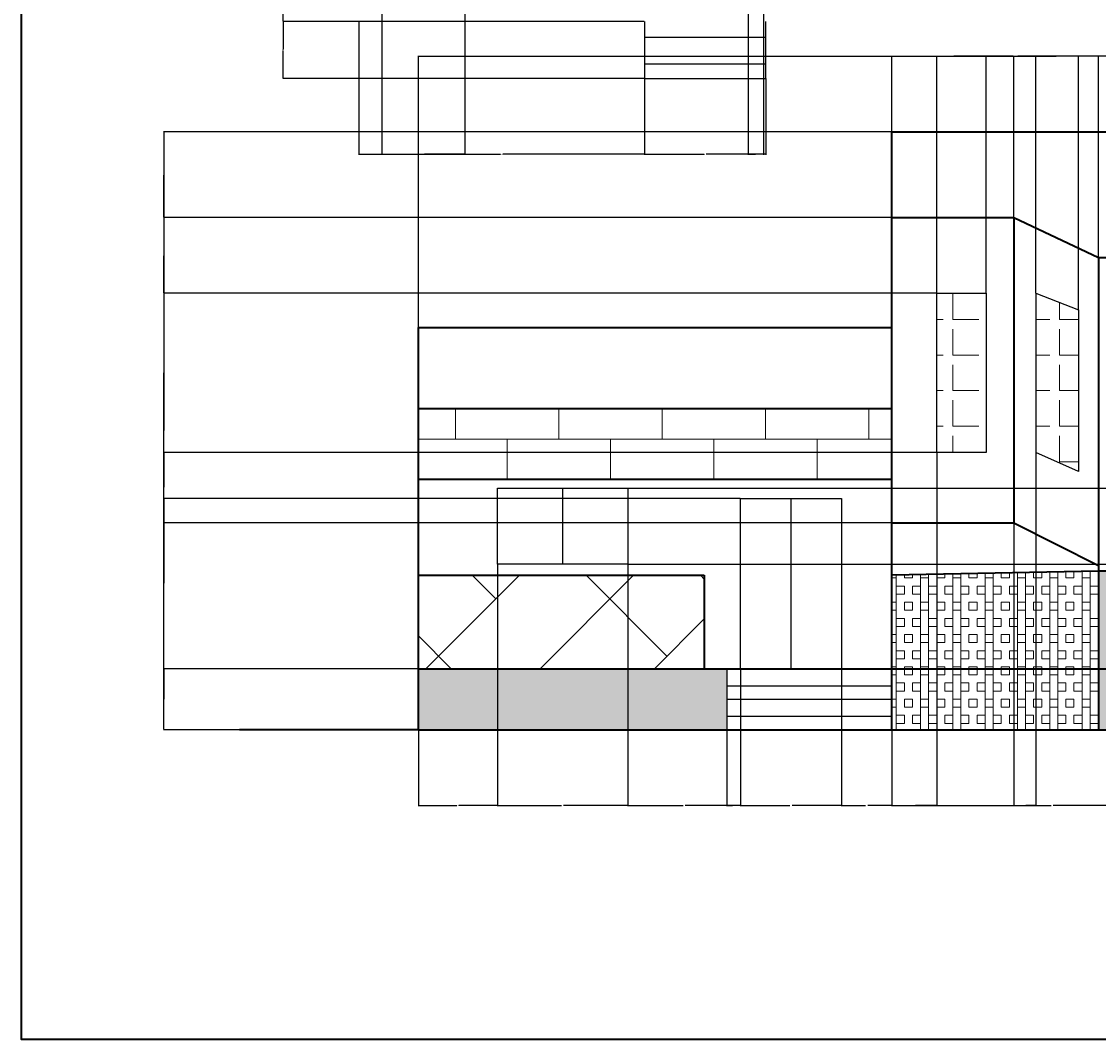
# Model space of a CAD drawing. Units: feet. Extents: x 3406 to 4127, y 2162 to 3204.
# Tile 1 of 3: x 3406 to 3829, y 2162 to 2562. Entities that reach past the tile are written whole.
import ezdxf

# ---------------------------------------------------------------- set-up
doc = ezdxf.new("R2010")
doc.units = ezdxf.units.FT
for name, color, linetype, lineweight in [('A-ANNO-DIMS', 2, 'Continuous', 18), ('A-ANNO-TTLB', 7, 'Continuous', 35), ('A-DOOR', 3, 'Continuous', 25), ('A-ELEV', 7, 'Continuous', 35), ('A-ELEV-GRND', 7, 'Continuous', 35), ('A-ELEV-PATT', 8, 'Continuous', 13), ('A-FLOR-STRS', 7, 'Continuous', 25), ('A-GLAZ', 4, 'Continuous', 25), ('A-GLAZ-PATT', 9, 'Continuous', 13)]:
    doc.layers.add(name, color=color, linetype=linetype, lineweight=lineweight)
doc.styles.get("Standard").update_dxf_attribs({"font": 'arial.ttf'})
doc.dimstyles.get("Standard").update_dxf_attribs({"dimtxt": 0.18, "dimasz": 0.18, "dimexe": 0.18, "dimexo": 0.0625, "dimgap": 0.09, "dimtad": 0, "dimtih": 1, "dimtoh": 1, "dimdec": 4, "dimzin": 0, "dimdsep": 46, "dimtxsty": 'Standard', "dimcen": 0.09, "dimadec": 0, "dimazin": 0, "dimtfac": 1, "dimtdec": 4, "dimtofl": 0, "dimtmove": 0, "dimatfit": 3, "dimfxl": 1, "dimtolj": 1, "dimtzin": 0, "dimarcsym": 0})

# ---------------------------------------------------------------- blocks, each defined once
blk = doc.blocks.new('*D5')
at = {"layer": 'A-ANNO-DIMS', "color": 0, "lineweight": -2, "transparency": 16777216}
for p, q in [((3538.33, 3101.91), (3508.41, 3101.91)), ((3508.59, 3101.73), (3508.59, 2832.09)), ((3508.59, 2562.09), (3508.59, 2831.72)), ((3538.33, 2561.91), (3508.41, 2561.91))]:
    blk.add_line(p, q, dxfattribs=at)
at = {"layer": 'A-ANNO-DIMS', "color": 0, "transparency": 16777216}
for points in [[(3508.56, 3101.73), (3508.62, 3101.73), (3508.59, 3101.91)], [(3508.56, 2562.09), (3508.62, 2562.09), (3508.59, 2561.91)]]:
    blk.add_solid(points, dxfattribs=at)
at = {"layer": 'Defpoints', "color": 0, "transparency": 16777216}
for p in [(3538.39, 3101.91), (3508.59, 2561.91), (3538.39, 2561.91)]:
    blk.add_point(p, dxfattribs=at)
at = {"layer": 'A-ANNO-DIMS', "color": 0, "transparency": 16777216, "insert": (3508.59, 2831.91), "char_height": 0.18, "attachment_point": 5}
blk.add_mtext('\\A1;540', dxfattribs=at)
blk = doc.blocks.new('*D6')
at = {"layer": 'A-ANNO-DIMS', "color": 0, "lineweight": -2, "transparency": 16777216}
for p, q in [((3650.56, 2561.91), (3508.41, 2561.91)), ((3508.59, 2561.73), (3508.59, 2550.9)), ((3508.59, 2539.7), (3508.59, 2550.53)), ((3650.56, 2539.52), (3508.41, 2539.52))]:
    blk.add_line(p, q, dxfattribs=at)
at = {"layer": 'A-ANNO-DIMS', "color": 0, "transparency": 16777216}
for points in [[(3508.56, 2561.73), (3508.62, 2561.73), (3508.59, 2561.91)], [(3508.56, 2539.7), (3508.62, 2539.7), (3508.59, 2539.52)]]:
    blk.add_solid(points, dxfattribs=at)
at = {"layer": 'Defpoints', "color": 0, "transparency": 16777216}
for p in [(3508.59, 2561.91), (3650.62, 2561.91), (3650.62, 2539.52)]:
    blk.add_point(p, dxfattribs=at)
at = {"layer": 'A-ANNO-DIMS', "color": 0, "transparency": 16777216, "insert": (3508.59, 2550.71), "char_height": 0.18, "attachment_point": 5}
blk.add_mtext('\\A1;22.383', dxfattribs=at)
blk = doc.blocks.new('*D7')
at = {"layer": 'A-ANNO-DIMS', "color": 0, "lineweight": -2, "transparency": 16777216}
for p, q in [((3538.39, 2561.84), (3538.39, 2509.54)), ((3650.62, 2539.46), (3650.62, 2509.54)), ((3538.57, 2509.72), (3594.05, 2509.72)), ((3650.44, 2509.72), (3594.96, 2509.72))]:
    blk.add_line(p, q, dxfattribs=at)
at = {"layer": 'A-ANNO-DIMS', "color": 0, "transparency": 16777216}
for points in [[(3538.57, 2509.75), (3538.57, 2509.69), (3538.39, 2509.72)], [(3650.44, 2509.75), (3650.44, 2509.69), (3650.62, 2509.72)]]:
    blk.add_solid(points, dxfattribs=at)
at = {"layer": 'Defpoints', "color": 0, "transparency": 16777216}
for p in [(3538.39, 2561.91), (3650.62, 2539.52), (3650.62, 2509.72)]:
    blk.add_point(p, dxfattribs=at)
at = {"layer": 'A-ANNO-DIMS', "color": 0, "transparency": 16777216, "insert": (3594.51, 2509.72), "char_height": 0.18, "attachment_point": 5}
blk.add_mtext('\\A1;112.23', dxfattribs=at)
blk = doc.blocks.new('*D8')
at = {"layer": 'A-ANNO-DIMS', "color": 0, "lineweight": -2, "transparency": 16777216}
for p, q in [((3650.62, 2539.46), (3650.62, 2509.54)), ((3698.33, 2539.46), (3698.33, 2509.54)), ((3650.8, 2509.72), (3674.09, 2509.72)), ((3698.15, 2509.72), (3674.85, 2509.72))]:
    blk.add_line(p, q, dxfattribs=at)
at = {"layer": 'A-ANNO-DIMS', "color": 0, "transparency": 16777216}
for points in [[(3650.8, 2509.75), (3650.8, 2509.69), (3650.62, 2509.72)], [(3698.15, 2509.75), (3698.15, 2509.69), (3698.33, 2509.72)]]:
    blk.add_solid(points, dxfattribs=at)
at = {"layer": 'Defpoints', "color": 0, "transparency": 16777216}
for p in [(3650.62, 2539.52), (3698.33, 2539.52), (3698.33, 2509.72)]:
    blk.add_point(p, dxfattribs=at)
at = {"layer": 'A-ANNO-DIMS', "color": 0, "transparency": 16777216, "insert": (3674.47, 2509.72), "char_height": 0.18, "attachment_point": 5}
blk.add_mtext('\\A1;47.71', dxfattribs=at)
blk = doc.blocks.new('*D23')
at = {"layer": 'A-ANNO-DIMS', "color": 0, "lineweight": -2, "transparency": 16777216}
for p, q in [((3691.39, 3092.84), (3691.39, 2509.54)), ((3697.39, 3092.84), (3697.39, 2509.54)), ((3691.57, 2509.72), (3694.24, 2509.72)), ((3697.21, 2509.72), (3694.54, 2509.72))]:
    blk.add_line(p, q, dxfattribs=at)
at = {"layer": 'A-ANNO-DIMS', "color": 0, "transparency": 16777216}
for points in [[(3691.57, 2509.75), (3691.57, 2509.69), (3691.39, 2509.72)], [(3697.21, 2509.75), (3697.21, 2509.69), (3697.39, 2509.72)]]:
    blk.add_solid(points, dxfattribs=at)
at = {"layer": 'Defpoints', "color": 0, "transparency": 16777216}
for p in [(3691.39, 3092.91), (3697.39, 3092.91), (3697.39, 2509.72)]:
    blk.add_point(p, dxfattribs=at)
at = {"layer": 'A-ANNO-DIMS', "color": 0, "transparency": 16777216, "insert": (3694.39, 2509.72), "char_height": 0.18, "attachment_point": 5}
blk.add_mtext('\\A1;6', dxfattribs=at)
blk = doc.blocks.new('*D24')
at = {"layer": 'A-ANNO-DIMS', "color": 0, "lineweight": -2, "transparency": 16777216}
for p, q in [((3547.39, 2989.54), (3547.39, 2509.54)), ((3580.04, 2989.54), (3580.04, 2509.54)), ((3547.57, 2509.72), (3563.25, 2509.72)), ((3579.86, 2509.72), (3564.18, 2509.72))]:
    blk.add_line(p, q, dxfattribs=at)
at = {"layer": 'A-ANNO-DIMS', "color": 0, "transparency": 16777216}
for points in [[(3547.57, 2509.75), (3547.57, 2509.69), (3547.39, 2509.72)], [(3579.86, 2509.75), (3579.86, 2509.69), (3580.04, 2509.72)]]:
    blk.add_solid(points, dxfattribs=at)
at = {"layer": 'Defpoints', "color": 0, "transparency": 16777216}
for p in [(3547.39, 2989.6), (3580.04, 2989.6), (3580.04, 2509.72)]:
    blk.add_point(p, dxfattribs=at)
at = {"layer": 'A-ANNO-DIMS', "color": 0, "transparency": 16777216, "insert": (3563.71, 2509.72), "char_height": 0.18, "attachment_point": 5}
blk.add_mtext('\\A1;32.646', dxfattribs=at)
blk = doc.blocks.new('*D27')
at = {"layer": 'A-ANNO-DIMS', "color": 0, "lineweight": -2, "transparency": 16777216}
for p, q in [((3561.78, 2441.65), (3561.78, 2548.49)), ((3561.96, 2548.31), (3796.68, 2548.31)), ((4032.19, 2548.31), (3797.47, 2548.31)), ((4032.37, 2441.65), (4032.37, 2548.49))]:
    blk.add_line(p, q, dxfattribs=at)
at = {"layer": 'A-ANNO-DIMS', "color": 0, "transparency": 16777216}
for points in [[(3561.96, 2548.34), (3561.96, 2548.28), (3561.78, 2548.31)], [(4032.19, 2548.34), (4032.19, 2548.28), (4032.37, 2548.31)]]:
    blk.add_solid(points, dxfattribs=at)
at = {"layer": 'Defpoints', "color": 0, "transparency": 16777216}
for p in [(4032.37, 2548.31), (3561.78, 2441.59), (4032.37, 2441.59)]:
    blk.add_point(p, dxfattribs=at)
at = {"layer": 'A-ANNO-DIMS', "color": 0, "transparency": 16777216, "insert": (3797.08, 2548.31), "char_height": 0.18, "attachment_point": 5}
blk.add_mtext('\\A1;470.6', dxfattribs=at)
blk = doc.blocks.new('*D28')
at = {"layer": 'A-ANNO-DIMS', "color": 0, "lineweight": -2, "transparency": 16777216}
for p, q in [((3747.81, 2518.51), (3461.48, 2518.51)), ((3461.66, 2518.33), (3461.66, 2401.18)), ((3461.66, 2283.67), (3461.66, 2400.82)), ((3561.72, 2283.49), (3461.48, 2283.49))]:
    blk.add_line(p, q, dxfattribs=at)
at = {"layer": 'A-ANNO-DIMS', "color": 0, "transparency": 16777216}
for points in [[(3461.63, 2518.33), (3461.69, 2518.33), (3461.66, 2518.51)], [(3461.63, 2283.67), (3461.69, 2283.67), (3461.66, 2283.49)]]:
    blk.add_solid(points, dxfattribs=at)
at = {"layer": 'Defpoints', "color": 0, "transparency": 16777216}
for p in [(3747.88, 2518.51), (3461.66, 2283.49), (3561.78, 2283.49)]:
    blk.add_point(p, dxfattribs=at)
at = {"layer": 'A-ANNO-DIMS', "color": 0, "transparency": 16777216, "insert": (3461.66, 2401), "char_height": 0.18, "attachment_point": 5}
blk.add_mtext('\\A1;235', dxfattribs=at)
blk = doc.blocks.new('*D29')
at = {"layer": 'A-ANNO-DIMS', "color": 0, "lineweight": -2, "transparency": 16777216}
for p, q in [((3592.86, 2348.49), (3592.86, 2253.51)), ((3561.78, 2283.42), (3561.78, 2253.51)), ((3561.96, 2253.69), (3576.92, 2253.69)), ((3592.68, 2253.69), (3577.71, 2253.69))]:
    blk.add_line(p, q, dxfattribs=at)
at = {"layer": 'A-ANNO-DIMS', "color": 0, "transparency": 16777216}
for points in [[(3561.96, 2253.72), (3561.96, 2253.66), (3561.78, 2253.69)], [(3592.68, 2253.72), (3592.68, 2253.66), (3592.86, 2253.69)]]:
    blk.add_solid(points, dxfattribs=at)
at = {"layer": 'Defpoints', "color": 0, "transparency": 16777216}
for p in [(3592.86, 2348.55), (3561.78, 2283.49), (3592.86, 2253.69)]:
    blk.add_point(p, dxfattribs=at)
at = {"layer": 'A-ANNO-DIMS', "color": 0, "transparency": 16777216, "insert": (3577.32, 2253.69), "char_height": 0.18, "attachment_point": 5}
blk.add_mtext('\\A1;31.08', dxfattribs=at)
blk = doc.blocks.new('*D30')
at = {"layer": 'A-ANNO-DIMS', "color": 0, "lineweight": -2, "transparency": 16777216}
for p, q in [((3592.86, 2348.49), (3592.86, 2253.51)), ((3644.04, 2348.49), (3644.04, 2253.51)), ((3593.04, 2253.69), (3618.05, 2253.69)), ((3643.86, 2253.69), (3618.84, 2253.69))]:
    blk.add_line(p, q, dxfattribs=at)
at = {"layer": 'A-ANNO-DIMS', "color": 0, "transparency": 16777216}
for points in [[(3593.04, 2253.72), (3593.04, 2253.66), (3592.86, 2253.69)], [(3643.86, 2253.72), (3643.86, 2253.66), (3644.04, 2253.69)]]:
    blk.add_solid(points, dxfattribs=at)
at = {"layer": 'Defpoints', "color": 0, "transparency": 16777216}
for p in [(3592.86, 2348.55), (3644.04, 2348.55), (3644.04, 2253.69)]:
    blk.add_point(p, dxfattribs=at)
at = {"layer": 'A-ANNO-DIMS', "color": 0, "transparency": 16777216, "insert": (3618.45, 2253.69), "char_height": 0.18, "attachment_point": 5}
blk.add_mtext('\\A1;51.19', dxfattribs=at)
blk = doc.blocks.new('*D31')
at = {"layer": 'A-ANNO-DIMS', "color": 0, "lineweight": -2, "transparency": 16777216}
for p, q in [((3644.04, 2348.49), (3644.04, 2253.51)), ((3688.4, 2307.43), (3688.4, 2253.51)), ((3644.22, 2253.69), (3665.82, 2253.69)), ((3688.22, 2253.69), (3666.62, 2253.69))]:
    blk.add_line(p, q, dxfattribs=at)
at = {"layer": 'A-ANNO-DIMS', "color": 0, "transparency": 16777216}
for points in [[(3644.22, 2253.72), (3644.22, 2253.66), (3644.04, 2253.69)], [(3688.22, 2253.72), (3688.22, 2253.66), (3688.4, 2253.69)]]:
    blk.add_solid(points, dxfattribs=at)
at = {"layer": 'Defpoints', "color": 0, "transparency": 16777216}
for p in [(3644.04, 2348.55), (3688.4, 2307.5), (3688.4, 2253.69)]:
    blk.add_point(p, dxfattribs=at)
at = {"layer": 'A-ANNO-DIMS', "color": 0, "transparency": 16777216, "insert": (3666.22, 2253.69), "char_height": 0.18, "attachment_point": 5}
blk.add_mtext('\\A1;44.36', dxfattribs=at)
blk = doc.blocks.new('*D32')
at = {"layer": 'A-ANNO-DIMS', "color": 0, "lineweight": -2, "transparency": 16777216}
for p, q in [((3688.4, 2307.43), (3688.4, 2253.51)), ((3728.08, 2307.43), (3728.08, 2253.51)), ((3688.58, 2253.69), (3707.78, 2253.69)), ((3727.9, 2253.69), (3708.7, 2253.69))]:
    blk.add_line(p, q, dxfattribs=at)
at = {"layer": 'A-ANNO-DIMS', "color": 0, "transparency": 16777216}
for points in [[(3688.58, 2253.72), (3688.58, 2253.66), (3688.4, 2253.69)], [(3727.9, 2253.72), (3727.9, 2253.66), (3728.08, 2253.69)]]:
    blk.add_solid(points, dxfattribs=at)
at = {"layer": 'Defpoints', "color": 0, "transparency": 16777216}
for p in [(3688.4, 2307.5), (3728.08, 2307.5), (3728.08, 2253.69)]:
    blk.add_point(p, dxfattribs=at)
at = {"layer": 'A-ANNO-DIMS', "color": 0, "transparency": 16777216, "insert": (3708.24, 2253.69), "char_height": 0.18, "attachment_point": 5}
blk.add_mtext('\\A1;39.685', dxfattribs=at)
blk = doc.blocks.new('*D33')
at = {"layer": 'A-ANNO-DIMS', "color": 0, "lineweight": -2, "transparency": 16777216}
for p, q in [((3728.08, 2307.43), (3728.08, 2253.51)), ((3747.88, 2283.42), (3747.88, 2253.51)), ((3728.26, 2253.69), (3737.53, 2253.69)), ((3747.7, 2253.69), (3738.43, 2253.69))]:
    blk.add_line(p, q, dxfattribs=at)
at = {"layer": 'A-ANNO-DIMS', "color": 0, "transparency": 16777216}
for points in [[(3728.26, 2253.72), (3728.26, 2253.66), (3728.08, 2253.69)], [(3747.7, 2253.72), (3747.7, 2253.66), (3747.88, 2253.69)]]:
    blk.add_solid(points, dxfattribs=at)
at = {"layer": 'Defpoints', "color": 0, "transparency": 16777216}
for p in [(3728.08, 2307.5), (3747.88, 2283.49), (3747.88, 2253.69)]:
    blk.add_point(p, dxfattribs=at)
at = {"layer": 'A-ANNO-DIMS', "color": 0, "transparency": 16777216, "insert": (3737.98, 2253.69), "char_height": 0.18, "attachment_point": 5}
blk.add_mtext('\\A1;19.794', dxfattribs=at)
blk = doc.blocks.new('*D34')
at = {"layer": 'A-ANNO-DIMS', "color": 0, "lineweight": -2, "transparency": 16777216}
for p, q in [((3747.88, 2283.42), (3747.88, 2253.51)), ((3874.08, 2283.42), (3874.08, 2253.51)), ((3748.06, 2253.69), (3810.59, 2253.69)), ((3873.9, 2253.69), (3811.36, 2253.69))]:
    blk.add_line(p, q, dxfattribs=at)
at = {"layer": 'A-ANNO-DIMS', "color": 0, "transparency": 16777216}
for points in [[(3748.06, 2253.72), (3748.06, 2253.66), (3747.88, 2253.69)], [(3873.9, 2253.72), (3873.9, 2253.66), (3874.08, 2253.69)]]:
    blk.add_solid(points, dxfattribs=at)
at = {"layer": 'Defpoints', "color": 0, "transparency": 16777216}
for p in [(3747.88, 2283.49), (3874.08, 2283.49), (3874.08, 2253.69)]:
    blk.add_point(p, dxfattribs=at)
at = {"layer": 'A-ANNO-DIMS', "color": 0, "transparency": 16777216, "insert": (3810.98, 2253.69), "char_height": 0.18, "attachment_point": 5}
blk.add_mtext('\\A1;126.2', dxfattribs=at)
blk = doc.blocks.new('*D37')
at = {"layer": 'A-ANNO-DIMS', "color": 0, "lineweight": -2, "transparency": 16777216}
for p, q in [((3682.91, 2307.5), (3461.48, 2307.5)), ((3461.66, 2307.32), (3461.66, 2295.67)), ((3461.66, 2283.67), (3461.66, 2295.31)), ((3682.91, 2283.49), (3461.48, 2283.49))]:
    blk.add_line(p, q, dxfattribs=at)
at = {"layer": 'A-ANNO-DIMS', "color": 0, "transparency": 16777216}
for points in [[(3461.63, 2307.32), (3461.69, 2307.32), (3461.66, 2307.5)], [(3461.63, 2283.67), (3461.69, 2283.67), (3461.66, 2283.49)]]:
    blk.add_solid(points, dxfattribs=at)
at = {"layer": 'Defpoints', "color": 0, "transparency": 16777216}
for p in [(3461.66, 2307.5), (3682.97, 2307.5), (3682.97, 2283.49)]:
    blk.add_point(p, dxfattribs=at)
at = {"layer": 'A-ANNO-DIMS', "color": 0, "transparency": 16777216, "insert": (3461.66, 2295.49), "char_height": 0.18, "attachment_point": 5}
blk.add_mtext('\\A1;24.01', dxfattribs=at)
blk = doc.blocks.new('*D38')
at = {"layer": 'A-ANNO-DIMS', "color": 0, "lineweight": -2, "transparency": 16777216}
for p, q in [((3688.4, 2307.43), (3688.4, 2253.51)), ((3682.97, 2283.42), (3682.97, 2253.51)), ((3683.15, 2253.69), (3685.29, 2253.69)), ((3688.22, 2253.69), (3686.08, 2253.69))]:
    blk.add_line(p, q, dxfattribs=at)
at = {"layer": 'A-ANNO-DIMS', "color": 0, "transparency": 16777216}
for points in [[(3683.15, 2253.72), (3683.15, 2253.66), (3682.97, 2253.69)], [(3688.22, 2253.72), (3688.22, 2253.66), (3688.4, 2253.69)]]:
    blk.add_solid(points, dxfattribs=at)
at = {"layer": 'Defpoints', "color": 0, "transparency": 16777216}
for p in [(3688.4, 2307.5), (3682.97, 2283.49), (3688.4, 2253.69)]:
    blk.add_point(p, dxfattribs=at)
at = {"layer": 'A-ANNO-DIMS', "color": 0, "transparency": 16777216, "insert": (3685.68, 2253.69), "char_height": 0.18, "attachment_point": 5}
blk.add_mtext('\\A1;5.427', dxfattribs=at)
blk = doc.blocks.new('*D39')
at = {"layer": 'A-ANNO-DIMS', "color": 0, "lineweight": -2, "transparency": 16777216}
for p, q in [((3688.34, 2374.42), (3461.48, 2374.42)), ((3461.66, 2374.24), (3461.66, 2341.14)), ((3461.66, 2307.68), (3461.66, 2340.78)), ((3688.34, 2307.5), (3461.48, 2307.5))]:
    blk.add_line(p, q, dxfattribs=at)
at = {"layer": 'A-ANNO-DIMS', "color": 0, "transparency": 16777216}
for points in [[(3461.63, 2374.24), (3461.69, 2374.24), (3461.66, 2374.42)], [(3461.63, 2307.68), (3461.69, 2307.68), (3461.66, 2307.5)]]:
    blk.add_solid(points, dxfattribs=at)
at = {"layer": 'Defpoints', "color": 0, "transparency": 16777216}
for p in [(3461.66, 2374.42), (3688.4, 2374.42), (3688.4, 2307.5)]:
    blk.add_point(p, dxfattribs=at)
at = {"layer": 'A-ANNO-DIMS', "color": 0, "transparency": 16777216, "insert": (3461.66, 2340.96), "char_height": 0.18, "attachment_point": 5}
blk.add_mtext('\\A1;66.93', dxfattribs=at)
blk = doc.blocks.new('*D42')
at = {"layer": 'A-ANNO-DIMS', "color": 0, "lineweight": -2, "transparency": 16777216}
for p, q in [((3644.1, 2378.49), (4100.86, 2378.49)), ((4100.68, 2378.31), (4100.68, 2363.7)), ((4100.68, 2348.73), (4100.68, 2363.34)), ((3644.1, 2348.55), (4100.86, 2348.55))]:
    blk.add_line(p, q, dxfattribs=at)
at = {"layer": 'A-ANNO-DIMS', "color": 0, "transparency": 16777216}
for points in [[(4100.65, 2378.31), (4100.71, 2378.31), (4100.68, 2378.49)], [(4100.65, 2348.73), (4100.71, 2348.73), (4100.68, 2348.55)]]:
    blk.add_solid(points, dxfattribs=at)
at = {"layer": 'Defpoints', "color": 0, "transparency": 16777216}
for p in [(3644.04, 2378.49), (4100.68, 2378.49), (3644.04, 2348.55)]:
    blk.add_point(p, dxfattribs=at)
at = {"layer": 'A-ANNO-DIMS', "color": 0, "transparency": 16777216, "insert": (4100.68, 2363.52), "char_height": 0.18, "attachment_point": 5}
blk.add_mtext('\\A1;29.935', dxfattribs=at)
blk = doc.blocks.new('*D43')
at = {"layer": 'A-ANNO-DIMS', "color": 0, "lineweight": -2, "transparency": 16777216}
for p, q in [((3644.1, 2348.55), (4100.86, 2348.55)), ((4100.68, 2348.37), (4100.68, 2328.21)), ((4100.68, 2307.68), (4100.68, 2327.84)), ((3674.17, 2307.5), (4100.86, 2307.5))]:
    blk.add_line(p, q, dxfattribs=at)
at = {"layer": 'A-ANNO-DIMS', "color": 0, "transparency": 16777216}
for points in [[(4100.65, 2348.37), (4100.71, 2348.37), (4100.68, 2348.55)], [(4100.65, 2307.68), (4100.71, 2307.68), (4100.68, 2307.5)]]:
    blk.add_solid(points, dxfattribs=at)
at = {"layer": 'Defpoints', "color": 0, "transparency": 16777216}
for p in [(3644.04, 2348.55), (3674.11, 2307.5), (4100.68, 2307.5)]:
    blk.add_point(p, dxfattribs=at)
at = {"layer": 'A-ANNO-DIMS', "color": 0, "transparency": 16777216, "insert": (4100.68, 2328.02), "char_height": 0.18, "attachment_point": 5}
blk.add_mtext('\\A1;41.055', dxfattribs=at)
blk = doc.blocks.new('*D44')
at = {"layer": 'A-ANNO-DIMS', "color": 0, "lineweight": -2, "transparency": 16777216}
for p, q in [((3747.88, 2484.91), (3747.88, 2548.49)), ((3748.06, 2548.31), (3771.46, 2548.31)), ((3795.66, 2548.31), (3772.26, 2548.31)), ((3795.84, 2484.91), (3795.84, 2548.49))]:
    blk.add_line(p, q, dxfattribs=at)
at = {"layer": 'A-ANNO-DIMS', "color": 0, "transparency": 16777216}
for points in [[(3748.06, 2548.34), (3748.06, 2548.28), (3747.88, 2548.31)], [(3795.66, 2548.34), (3795.66, 2548.28), (3795.84, 2548.31)]]:
    blk.add_solid(points, dxfattribs=at)
at = {"layer": 'Defpoints', "color": 0, "transparency": 16777216}
for p in [(3795.84, 2548.31), (3747.88, 2484.85), (3795.84, 2484.85)]:
    blk.add_point(p, dxfattribs=at)
at = {"layer": 'A-ANNO-DIMS', "color": 0, "transparency": 16777216, "insert": (3771.86, 2548.31), "char_height": 0.18, "attachment_point": 5}
blk.add_mtext('\\A1;47.97', dxfattribs=at)
blk = doc.blocks.new('*D45')
at = {"layer": 'A-ANNO-DIMS', "color": 0, "lineweight": -2, "transparency": 16777216}
for p, q in [((3795.84, 2484.91), (3795.84, 2548.49)), ((3796.02, 2548.31), (3812.11, 2548.31)), ((3828.99, 2548.31), (3812.9, 2548.31)), ((3829.17, 2469.25), (3829.17, 2548.49))]:
    blk.add_line(p, q, dxfattribs=at)
at = {"layer": 'A-ANNO-DIMS', "color": 0, "transparency": 16777216}
for points in [[(3796.02, 2548.34), (3796.02, 2548.28), (3795.84, 2548.31)], [(3828.99, 2548.34), (3828.99, 2548.28), (3829.17, 2548.31)]]:
    blk.add_solid(points, dxfattribs=at)
at = {"layer": 'Defpoints', "color": 0, "transparency": 16777216}
for p in [(3829.17, 2548.31), (3795.84, 2484.85), (3829.17, 2469.19)]:
    blk.add_point(p, dxfattribs=at)
at = {"layer": 'A-ANNO-DIMS', "color": 0, "transparency": 16777216, "insert": (3812.51, 2548.31), "char_height": 0.18, "attachment_point": 5}
blk.add_mtext('\\A1;33.32', dxfattribs=at)
blk = doc.blocks.new('*D46')
at = {"layer": 'A-ANNO-DIMS', "color": 0, "lineweight": -2, "transparency": 16777216}
for p, q in [((3765.67, 2392.47), (3765.67, 2253.51)), ((3747.88, 2364.79), (3747.88, 2253.51)), ((3748.06, 2253.69), (3756.39, 2253.69)), ((3765.49, 2253.69), (3757.16, 2253.69))]:
    blk.add_line(p, q, dxfattribs=at)
at = {"layer": 'A-ANNO-DIMS', "color": 0, "transparency": 16777216}
for points in [[(3748.06, 2253.72), (3748.06, 2253.66), (3747.88, 2253.69)], [(3765.49, 2253.72), (3765.49, 2253.66), (3765.67, 2253.69)]]:
    blk.add_solid(points, dxfattribs=at)
at = {"layer": 'Defpoints', "color": 0, "transparency": 16777216}
for p in [(3765.67, 2392.53), (3747.88, 2364.85), (3765.67, 2253.69)]:
    blk.add_point(p, dxfattribs=at)
at = {"layer": 'A-ANNO-DIMS', "color": 0, "transparency": 16777216, "insert": (3756.77, 2253.69), "char_height": 0.18, "attachment_point": 5}
blk.add_mtext('\\A1;17.79', dxfattribs=at)
blk = doc.blocks.new('*D47')
at = {"layer": 'A-ANNO-DIMS', "color": 0, "lineweight": -2, "transparency": 16777216}
for p, q in [((3765.67, 2455.14), (3765.67, 2548.49)), ((3765.85, 2548.31), (3774.91, 2548.31)), ((3784.89, 2548.31), (3775.82, 2548.31)), ((3785.07, 2455.14), (3785.07, 2548.49))]:
    blk.add_line(p, q, dxfattribs=at)
at = {"layer": 'A-ANNO-DIMS', "color": 0, "transparency": 16777216}
for points in [[(3765.85, 2548.34), (3765.85, 2548.28), (3765.67, 2548.31)], [(3784.89, 2548.34), (3784.89, 2548.28), (3785.07, 2548.31)]]:
    blk.add_solid(points, dxfattribs=at)
at = {"layer": 'Defpoints', "color": 0, "transparency": 16777216}
for p in [(3785.07, 2548.31), (3765.67, 2455.08), (3785.07, 2455.08)]:
    blk.add_point(p, dxfattribs=at)
at = {"layer": 'A-ANNO-DIMS', "color": 0, "transparency": 16777216, "insert": (3775.37, 2548.31), "char_height": 0.18, "attachment_point": 5}
blk.add_mtext('\\A1;19.397', dxfattribs=at)
blk = doc.blocks.new('*D48')
at = {"layer": 'A-ANNO-DIMS', "color": 0, "lineweight": -2, "transparency": 16777216}
for p, q in [((3804.58, 2392.47), (3804.58, 2253.51)), ((3795.84, 2364.79), (3795.84, 2253.51)), ((3796.02, 2253.69), (3799.82, 2253.69)), ((3804.4, 2253.69), (3800.61, 2253.69))]:
    blk.add_line(p, q, dxfattribs=at)
at = {"layer": 'A-ANNO-DIMS', "color": 0, "transparency": 16777216}
for points in [[(3796.02, 2253.72), (3796.02, 2253.66), (3795.84, 2253.69)], [(3804.4, 2253.72), (3804.4, 2253.66), (3804.58, 2253.69)]]:
    blk.add_solid(points, dxfattribs=at)
at = {"layer": 'Defpoints', "color": 0, "transparency": 16777216}
for p in [(3804.58, 2392.53), (3795.84, 2364.85), (3804.58, 2253.69)]:
    blk.add_point(p, dxfattribs=at)
at = {"layer": 'A-ANNO-DIMS', "color": 0, "transparency": 16777216, "insert": (3800.21, 2253.69), "char_height": 0.18, "attachment_point": 5}
blk.add_mtext('\\A1;8.735', dxfattribs=at)
blk = doc.blocks.new('*D49')
at = {"layer": 'A-ANNO-DIMS', "color": 0, "lineweight": -2, "transparency": 16777216}
for p, q in [((3804.58, 2455.14), (3804.58, 2548.49)), ((3804.76, 2548.31), (3812.56, 2548.31)), ((3821.13, 2548.31), (3813.33, 2548.31)), ((3821.31, 2448.6), (3821.31, 2548.49))]:
    blk.add_line(p, q, dxfattribs=at)
at = {"layer": 'A-ANNO-DIMS', "color": 0, "transparency": 16777216}
for points in [[(3804.76, 2548.34), (3804.76, 2548.28), (3804.58, 2548.31)], [(3821.13, 2548.34), (3821.13, 2548.28), (3821.31, 2548.31)]]:
    blk.add_solid(points, dxfattribs=at)
at = {"layer": 'Defpoints', "color": 0, "transparency": 16777216}
for p in [(3821.31, 2548.31), (3804.58, 2455.08), (3821.31, 2448.54)]:
    blk.add_point(p, dxfattribs=at)
at = {"layer": 'A-ANNO-DIMS', "color": 0, "transparency": 16777216, "insert": (3812.94, 2548.31), "char_height": 0.18, "attachment_point": 5}
blk.add_mtext('\\A1;16.73', dxfattribs=at)
blk = doc.blocks.new('*D52')
at = {"layer": 'A-ANNO-DIMS', "color": 0, "lineweight": -2, "transparency": 16777216}
for p, q in [((3747.81, 2518.51), (3461.48, 2518.51)), ((3461.66, 2518.33), (3461.66, 2501.86)), ((3461.66, 2485.03), (3461.66, 2501.5)), ((3747.81, 2484.85), (3461.48, 2484.85))]:
    blk.add_line(p, q, dxfattribs=at)
at = {"layer": 'A-ANNO-DIMS', "color": 0, "transparency": 16777216}
for points in [[(3461.63, 2518.33), (3461.69, 2518.33), (3461.66, 2518.51)], [(3461.63, 2485.03), (3461.69, 2485.03), (3461.66, 2484.85)]]:
    blk.add_solid(points, dxfattribs=at)
at = {"layer": 'Defpoints', "color": 0, "transparency": 16777216}
for p in [(3747.88, 2518.51), (3461.66, 2484.85), (3747.88, 2484.85)]:
    blk.add_point(p, dxfattribs=at)
at = {"layer": 'A-ANNO-DIMS', "color": 0, "transparency": 16777216, "insert": (3461.66, 2501.68), "char_height": 0.18, "attachment_point": 5}
blk.add_mtext('\\A1;33.66', dxfattribs=at)
blk = doc.blocks.new('*D53')
at = {"layer": 'A-ANNO-DIMS', "color": 0, "lineweight": -2, "transparency": 16777216}
for p, q in [((3747.81, 2484.85), (3461.48, 2484.85)), ((3461.66, 2484.67), (3461.66, 2470.15)), ((3461.66, 2455.26), (3461.66, 2469.78)), ((3765.61, 2455.08), (3461.48, 2455.08))]:
    blk.add_line(p, q, dxfattribs=at)
at = {"layer": 'A-ANNO-DIMS', "color": 0, "transparency": 16777216}
for points in [[(3461.63, 2484.67), (3461.69, 2484.67), (3461.66, 2484.85)], [(3461.63, 2455.26), (3461.69, 2455.26), (3461.66, 2455.08)]]:
    blk.add_solid(points, dxfattribs=at)
at = {"layer": 'Defpoints', "color": 0, "transparency": 16777216}
for p in [(3747.88, 2484.85), (3461.66, 2455.08), (3765.67, 2455.08)]:
    blk.add_point(p, dxfattribs=at)
at = {"layer": 'A-ANNO-DIMS', "color": 0, "transparency": 16777216, "insert": (3461.66, 2469.97), "char_height": 0.18, "attachment_point": 5}
blk.add_mtext('\\A1;29.77', dxfattribs=at)
blk = doc.blocks.new('*D54')
at = {"layer": 'A-ANNO-DIMS', "color": 0, "lineweight": -2, "transparency": 16777216}
for p, q in [((3765.61, 2455.08), (3461.48, 2455.08)), ((3461.66, 2454.9), (3461.66, 2423.99)), ((3461.66, 2392.71), (3461.66, 2423.62)), ((3765.61, 2392.53), (3461.48, 2392.53))]:
    blk.add_line(p, q, dxfattribs=at)
at = {"layer": 'A-ANNO-DIMS', "color": 0, "transparency": 16777216}
for points in [[(3461.63, 2454.9), (3461.69, 2454.9), (3461.66, 2455.08)], [(3461.63, 2392.71), (3461.69, 2392.71), (3461.66, 2392.53)]]:
    blk.add_solid(points, dxfattribs=at)
at = {"layer": 'Defpoints', "color": 0, "transparency": 16777216}
for p in [(3765.67, 2455.08), (3461.66, 2392.53), (3765.67, 2392.53)]:
    blk.add_point(p, dxfattribs=at)
at = {"layer": 'A-ANNO-DIMS', "color": 0, "transparency": 16777216, "insert": (3461.66, 2423.81), "char_height": 0.18, "attachment_point": 5}
blk.add_mtext('\\A1;62.55', dxfattribs=at)
blk = doc.blocks.new('*D55')
at = {"layer": 'A-ANNO-DIMS', "color": 0, "lineweight": -2, "transparency": 16777216}
for p, q in [((3765.61, 2392.53), (3461.48, 2392.53)), ((3461.66, 2392.35), (3461.66, 2378.87)), ((3461.66, 2365.03), (3461.66, 2378.51)), ((3747.81, 2364.85), (3461.48, 2364.85))]:
    blk.add_line(p, q, dxfattribs=at)
at = {"layer": 'A-ANNO-DIMS', "color": 0, "transparency": 16777216}
for points in [[(3461.63, 2392.35), (3461.69, 2392.35), (3461.66, 2392.53)], [(3461.63, 2365.03), (3461.69, 2365.03), (3461.66, 2364.85)]]:
    blk.add_solid(points, dxfattribs=at)
at = {"layer": 'Defpoints', "color": 0, "transparency": 16777216}
for p in [(3765.67, 2392.53), (3461.66, 2364.85), (3747.88, 2364.85)]:
    blk.add_point(p, dxfattribs=at)
at = {"layer": 'A-ANNO-DIMS', "color": 0, "transparency": 16777216, "insert": (3461.66, 2378.69), "char_height": 0.18, "attachment_point": 5}
blk.add_mtext('\\A1;27.683', dxfattribs=at)

msp = doc.modelspace()

# ---------------------------------------------------------------- hatches: boundary and pattern name
at = {"layer": 'A-ELEV-PATT'}
h = msp.add_hatch(dxfattribs=at)
h.set_pattern_fill('AR-B816', color=256, scale=0.1)
h.paths.add_polyline_path([(3747.8769, 2409.819), (3561.7785, 2409.819), (3561.7785, 2382.0333), (3747.8769, 2382.0333)])
h.paths.add_polyline_path([(4032.3722, 2412.4251), (3874.0816, 2412.4251), (3874.0816, 2382.0333), (4032.3722, 2382.0333)])
h = msp.add_hatch(dxfattribs=at)
h.set_pattern_fill('BRICK', color=256, scale=0.5)
h.paths.add_polyline_path([(3874.0816, 2345.984), (3829.1663, 2345.984), (3829.1663, 2307.4958), (3874.0816, 2307.4958)])
h.paths.add_polyline_path([(3874.0816, 2307.4958), (3829.1663, 2307.4958), (3829.1663, 2283.4863), (3874.0816, 2283.4863)])
h.paths.add_polyline_path([(4032.3722, 2307.4958), (3874.0816, 2307.4958), (3874.0816, 2283.4863), (4032.3722, 2283.4863)])
h.paths.add_polyline_path([(3682.9714, 2307.4958), (3561.7785, 2307.4958), (3561.7785, 2283.4863), (3682.9714, 2283.4863)])
h = msp.add_hatch(dxfattribs=at)
h.set_pattern_fill('ANSI38', color=256, scale=10)
h.paths.add_polyline_path([(3674.1115, 2344.2093), (3561.7785, 2344.2093), (3561.7785, 2307.4958), (3674.1115, 2307.4958)])
h = msp.add_hatch(dxfattribs=at)
h.set_pattern_fill('BOX', color=256, scale=0.5)
h.paths.add_polyline_path([(3829.1663, 2345.984), (3747.8769, 2344.3747), (3747.8769, 2307.4958), (3829.1663, 2307.4958)])
h.paths.add_polyline_path([(3829.1663, 2307.4958), (3747.8769, 2307.4958), (3747.8769, 2283.4863), (3829.1663, 2283.4863)])
at = {"layer": 'A-GLAZ-PATT'}
h = msp.add_hatch(dxfattribs=at)
h.set_pattern_fill('ANGLE', color=256, scale=2)
h.set_pattern_definition([(0, (0, 0), (0, 13.97), [10.16, -3.81]), (90, (0, 0), (-13.97, 9e-16), [10.16, -3.81])])
h.paths.add_polyline_path([(3866.4229, 2448.5363), (3840.6, 2448.5363), (3840.6, 2388.7978), (3866.4229, 2388.7978)])
h.paths.add_polyline_path([(3821.3093, 2448.5363), (3804.5796, 2455.082), (3804.5796, 2392.5307), (3821.3093, 2385.0649)])
h.paths.add_polyline_path([(3785.0653, 2455.082), (3765.6683, 2455.082), (3765.6683, 2392.5307), (3785.0653, 2392.5307)])

# ---------------------------------------------------------------- linework, layer by layer
at = {"layer": 'A-ANNO-TTLB'}
msp.add_lwpolyline([(3405.6917, 3203.7208), (4127.2965, 3203.7208), (4127.2965, 2161.7472), (3405.6917, 2161.7472)], close=True, dxfattribs=at)
at = {"layer": 'A-DOOR'}
msp.add_line((3708.2407, 2374.4234), (3708.2407, 2307.4958), dxfattribs=at)
msp.add_lwpolyline([(3688.3981, 2374.4234), (3728.0832, 2374.4234), (3728.0832, 2307.4958), (3688.3981, 2307.4958)], close=True, dxfattribs=at)
at = {"layer": 'A-ELEV'}
for p, q in [((3747.8769, 2283.4863), (3747.8769, 2518.5088)), ((3747.8769, 2518.5088), (3874.0816, 2518.5088)), ((3747.8769, 2484.8499), (3795.8441, 2484.8499)), ((3795.8441, 2484.8499), (3829.1663, 2469.1901)), ((3795.8441, 2484.8499), (3795.8441, 2364.8477)), ((3829.1663, 2469.1901), (3874.0816, 2469.1901)), ((3829.1663, 2469.1901), (3829.1663, 2345.984)), ((3561.7785, 2283.4863), (3561.7785, 2441.5924)), ((3561.7785, 2441.5924), (3747.8769, 2441.5924)), ((3561.7785, 2409.819), (3747.8769, 2409.819)), ((3561.7785, 2382.0333), (3747.8769, 2382.0333)), ((3747.8769, 2364.8477), (3795.8441, 2364.8477)), ((3795.8441, 2364.8477), (3829.1663, 2348.012)), ((3561.7785, 2344.2093), (3674.1115, 2344.2093)), ((3674.1115, 2344.2093), (3674.1115, 2307.4958)), ((3747.8769, 2344.3747), (3829.1663, 2345.984)), ((3829.1663, 2345.984), (3874.0816, 2345.984)), ((3829.1663, 2345.984), (3829.1663, 2283.4863)), ((3561.7785, 2307.4958), (4032.3722, 2307.4958))]:
    msp.add_line(p, q, dxfattribs=at)
at = {"layer": 'A-ELEV-GRND'}
for q in [(3491.4641, 2283.4863), (4070.8753, 2283.4863)]:
    msp.add_line((3561.7785, 2283.4863), q, dxfattribs=at)
at = {"layer": 'A-FLOR-STRS'}
for p, q in [((3650.6189, 2561.9057), (3650.6189, 2539.5223)), ((3698.33, 2539.5223), (3698.33, 2561.9057)), ((3650.6189, 2555.7949), (3698.33, 2555.7949)), ((3650.6189, 2545.334), (3698.33, 2545.334)), ((3650.6189, 2539.5223), (3698.33, 2539.5223)), ((3682.9714, 2307.4958), (3682.9714, 2283.4863)), ((3682.9714, 2300.8079), (3747.8769, 2300.8079)), ((3682.9714, 2295.491), (3747.8769, 2295.491)), ((3682.9714, 2288.849), (3747.8769, 2288.849))]:
    msp.add_line(p, q, dxfattribs=at)
at = {"layer": 'A-GLAZ'}
for p, q in [((3765.6683, 2455.082), (3785.0653, 2455.082)), ((3765.6683, 2392.5307), (3765.6683, 2455.082)), ((3785.0653, 2455.082), (3785.0653, 2392.5307)), ((3804.5796, 2455.082), (3804.5796, 2392.5307)), ((3804.5796, 2455.082), (3821.3093, 2448.5363)), ((3821.3093, 2448.5363), (3821.3093, 2385.0649)), ((3785.0653, 2392.5307), (3765.6683, 2392.5307)), ((3821.3093, 2385.0649), (3804.5796, 2392.5307)), ((3618.4485, 2378.4862), (3618.4485, 2348.5507))]:
    msp.add_line(p, q, dxfattribs=at)
msp.add_lwpolyline([(3592.8558, 2378.4862), (3644.0412, 2378.4862), (3644.0412, 2348.5507), (3592.8558, 2348.5507)], close=True, dxfattribs=at)

# ---------------------------------------------------------------- dimensions: what is measured, and where the dimension line sits
at = {"layer": 'A-ANNO-DIMS'}
for base, p1, p2, override, picture, middle in [((3508.5916, 2561.9057), (3538.3916, 3101.9057), (3538.3916, 2561.9057), {"dimdec": 0, "dimlfac": 1, "dimrnd": 0, "dimzin": 0, "dimdsep": 46, "dimlunit": 2}, '*D5', (3508.5916, 2831.9057)), ((3508.5916, 2561.9057), (3650.6189, 2539.5223), (3650.6189, 2561.9057), {"dimdec": 3, "dimlfac": 1, "dimrnd": 0, "dimzin": 0, "dimdsep": 46, "dimlunit": 2}, '*D6', (3508.5916, 2550.714)), ((3461.6641, 2484.8499), (3747.8769, 2518.5088), (3747.8769, 2484.8499), {"dimdec": 2, "dimlfac": 1, "dimrnd": 0, "dimzin": 0, "dimdsep": 46, "dimlunit": 2}, '*D52', (3461.6641, 2501.6794)), ((3461.6641, 2283.4863), (3747.8769, 2518.5088), (3561.7785, 2283.4863), {"dimdec": 0, "dimlfac": 1, "dimrnd": 0, "dimzin": 0, "dimdsep": 46, "dimlunit": 2}, '*D28', (3461.6641, 2400.9976)), ((3461.6641, 2455.082), (3747.8769, 2484.8499), (3765.6683, 2455.082), {"dimdec": 2, "dimlfac": 1, "dimrnd": 0, "dimzin": 0, "dimdsep": 46, "dimlunit": 2}, '*D53', (3461.6641, 2469.966)), ((3461.6641, 2392.5307), (3765.6683, 2455.082), (3765.6683, 2392.5307), {"dimdec": 2, "dimlfac": 1, "dimrnd": 0, "dimzin": 0, "dimdsep": 46, "dimlunit": 2}, '*D54', (3461.6641, 2423.8064)), ((3461.6641, 2364.8477), (3765.6683, 2392.5307), (3747.8769, 2364.8477), {"dimdec": 3, "dimlfac": 1, "dimrnd": 0, "dimzin": 0, "dimdsep": 46, "dimlunit": 2}, '*D55', (3461.6641, 2378.6892)), ((4100.67532, 2378.4862), (3644.0412, 2348.55074), (3644.0412, 2378.4862), {"dimdec": 3, "dimlfac": 1, "dimrnd": 0, "dimzin": 0, "dimdsep": 46, "dimlunit": 2}, '*D42', (4100.67532, 2363.51847)), ((3461.6641, 2374.4234), (3688.3981, 2307.4958), (3688.3981, 2374.4234), {"dimdec": 2, "dimlfac": 1, "dimrnd": 0, "dimzin": 0, "dimdsep": 46, "dimlunit": 2}, '*D39', (3461.6641, 2340.9596)), ((4100.6753, 2307.4958), (3644.0412, 2348.5507), (3674.1115, 2307.4958), {"dimdec": 3, "dimlfac": 1, "dimrnd": 0, "dimzin": 0, "dimdsep": 46, "dimlunit": 2}, '*D43', (4100.6753, 2328.0233)), ((3461.6641, 2307.4958), (3682.9714, 2283.4863), (3682.9714, 2307.4958), {"dimdec": 2, "dimlfac": 1, "dimrnd": 0, "dimzin": 0, "dimdsep": 46, "dimlunit": 2}, '*D37', (3461.6641, 2295.491))]:
    dim = msp.add_linear_dim(base=base, p1=p1, p2=p2, angle=90, dimstyle='Standard', override=override, dxfattribs=at)
    dim.commit()
    dim.dimension.update_dxf_attribs({"geometry": picture, "text_midpoint": middle})
for base, p1, p2, override, picture, middle in [((3697.3916, 2509.7223), (3691.3916, 3092.9057), (3697.3916, 3092.9057), {"dimdec": 0, "dimlfac": 1, "dimrnd": 0, "dimzin": 0, "dimdsep": 46, "dimlunit": 2}, '*D23', (3694.3916, 2509.7223)), ((3580.0374, 2509.7223), (3547.3916, 2989.6004), (3580.0374, 2989.6004), {"dimdec": 3, "dimlfac": 1, "dimrnd": 0, "dimzin": 0, "dimdsep": 46, "dimlunit": 2}, '*D24', (3563.7145, 2509.7223)), ((3650.6189, 2509.7223), (3538.3916, 2561.9057), (3650.6189, 2539.5223), {"dimdec": 2, "dimlfac": 1, "dimrnd": 0, "dimzin": 0, "dimdsep": 46, "dimlunit": 2}, '*D7', (3594.5053, 2509.7223)), ((4032.3722, 2548.3088), (3561.7785, 2441.5924), (4032.3722, 2441.5924), {"dimdec": 1, "dimlfac": 1, "dimrnd": 0, "dimzin": 0, "dimdsep": 46, "dimlunit": 2}, '*D27', (3797.0754, 2548.3088)), ((3795.8441, 2548.3088), (3747.8769, 2484.8499), (3795.8441, 2484.8499), {"dimdec": 2, "dimlfac": 1, "dimrnd": 0, "dimzin": 0, "dimdsep": 46, "dimlunit": 2}, '*D44', (3771.8605, 2548.3088)), ((3785.0653, 2548.3088), (3765.6683, 2455.082), (3785.0653, 2455.082), {"dimdec": 3, "dimlfac": 1, "dimrnd": 0, "dimzin": 0, "dimdsep": 46, "dimlunit": 2}, '*D47', (3775.3668, 2548.3088)), ((3829.1663, 2548.3088), (3795.8441, 2484.8499), (3829.1663, 2469.1901), {"dimdec": 2, "dimlfac": 1, "dimrnd": 0, "dimzin": 0, "dimdsep": 46, "dimlunit": 2}, '*D45', (3812.5052, 2548.3088)), ((3821.3093, 2548.3088), (3804.5796, 2455.082), (3821.3093, 2448.5363), {"dimdec": 2, "dimlfac": 1, "dimrnd": 0, "dimzin": 0, "dimdsep": 46, "dimlunit": 2}, '*D49', (3812.9445, 2548.3088)), ((3698.33, 2509.7223), (3650.6189, 2539.5223), (3698.33, 2539.5223), {"dimdec": 2, "dimlfac": 1, "dimrnd": 0, "dimzin": 0, "dimdsep": 46, "dimlunit": 2}, '*D8', (3674.4745, 2509.7223)), ((3765.6683, 2253.6863), (3747.8769, 2364.8477), (3765.6683, 2392.5307), {"dimdec": 2, "dimlfac": 1, "dimrnd": 0, "dimzin": 0, "dimdsep": 46, "dimlunit": 2}, '*D46', (3756.7726, 2253.6863)), ((3804.57958, 2253.68626), (3795.8441, 2364.84773), (3804.57958, 2392.53069), {"dimdec": 3, "dimlfac": 1, "dimrnd": 0, "dimzin": 0, "dimdsep": 46, "dimlunit": 2}, '*D48', (3800.21184, 2253.68626)), ((3592.8558, 2253.6863), (3561.7785, 2283.4863), (3592.8558, 2348.5507), {"dimdec": 2, "dimlfac": 1, "dimrnd": 0, "dimzin": 0, "dimdsep": 46, "dimlunit": 2}, '*D29', (3577.3172, 2253.6863)), ((3644.0412, 2253.6863), (3592.8558, 2348.5507), (3644.0412, 2348.5507), {"dimdec": 2, "dimlfac": 1, "dimrnd": 0, "dimzin": 0, "dimdsep": 46, "dimlunit": 2}, '*D30', (3618.4485, 2253.6863)), ((3688.3981, 2253.6863), (3644.0412, 2348.5507), (3688.3981, 2307.4958), {"dimdec": 2, "dimlfac": 1, "dimrnd": 0, "dimzin": 0, "dimdsep": 46, "dimlunit": 2}, '*D31', (3666.2197, 2253.6863)), ((3688.3981, 2253.6863), (3682.9714, 2283.4863), (3688.3981, 2307.4958), {"dimdec": 3, "dimlfac": 1, "dimrnd": 0, "dimzin": 0, "dimdsep": 46, "dimlunit": 2}, '*D38', (3685.6848, 2253.6863)), ((3728.0832, 2253.6863), (3688.3981, 2307.4958), (3728.0832, 2307.4958), {"dimdec": 3, "dimlfac": 1, "dimrnd": 0, "dimzin": 0, "dimdsep": 46, "dimlunit": 2}, '*D32', (3708.2407, 2253.6863)), ((3747.8769, 2253.6863), (3728.0832, 2307.4958), (3747.8769, 2283.4863), {"dimdec": 3, "dimlfac": 1, "dimrnd": 0, "dimzin": 0, "dimdsep": 46, "dimlunit": 2}, '*D33', (3737.9801, 2253.6863)), ((3874.0816, 2253.6863), (3747.8769, 2283.4863), (3874.0816, 2283.4863), {"dimdec": 1, "dimlfac": 1, "dimrnd": 0, "dimzin": 0, "dimdsep": 46, "dimlunit": 2}, '*D34', (3810.9793, 2253.6863))]:
    dim = msp.add_linear_dim(base=base, p1=p1, p2=p2, dimstyle='Standard', override=override, dxfattribs=at)
    dim.commit()
    dim.dimension.update_dxf_attribs({"geometry": picture, "text_midpoint": middle})

doc.saveas('drawing.dxf')
